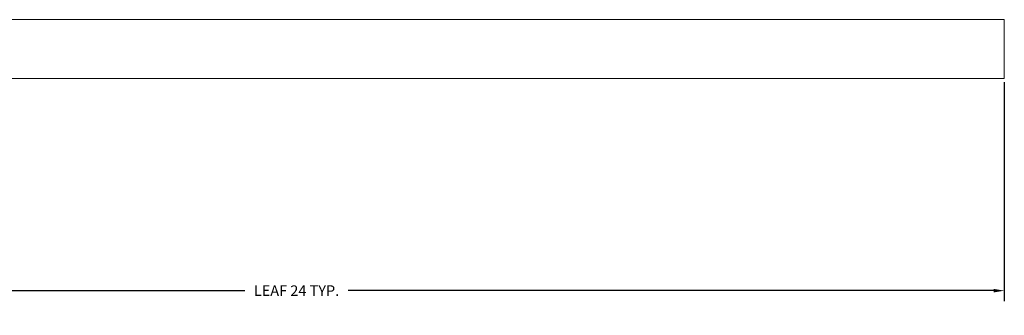
# Model space of a CAD drawing. Units: inches. Extents: x -86 to 2463, y -1058 to 68.
# Tile 7 of 17: x 32.07 to 48.76, y -277.59 to -272.57. Entities that reach past the tile are written whole.
import ezdxf

# ---------------------------------------------------------------- set-up
doc = ezdxf.new("R2010")
doc.units = ezdxf.units.IN
doc.header["$MEASUREMENT"] = 0
doc.layers.add('A-ANNO-DIMS', color=2, linetype='Continuous', lineweight=18)
doc.layers.add('A-DOOR', color=3, linetype='Continuous', lineweight=18)
doc.styles.get("Standard").update_dxf_attribs({"font": 'arial.ttf'})
doc.dimstyles.get("Standard").update_dxf_attribs({"dimtxt": 0.18, "dimasz": 0.18, "dimexe": 0.18, "dimexo": 0.0625, "dimgap": 0.09, "dimtad": 0, "dimtih": 1, "dimtoh": 1, "dimdec": 4, "dimzin": 0, "dimdsep": 46, "dimtxsty": 'Standard', "dimcen": 0.09, "dimadec": 0, "dimazin": 0, "dimtfac": 1, "dimtdec": 4, "dimtofl": 0, "dimtmove": 0, "dimatfit": 3, "dimfxl": 1, "dimtolj": 1, "dimtzin": 0, "dimarcsym": 0})

# ---------------------------------------------------------------- blocks, each defined once
blk = doc.blocks.new('DOOR-LEAF-24IN')
for p, q in [((0, 0), (0, 24)), ((0, 24), (1, 24)), ((1, 24), (1, 0)), ((1, 0), (0, 0))]:
    blk.add_line(p, q)
blk = doc.blocks.new('*D10')
at = {"layer": 'A-ANNO-DIMS', "color": 0, "lineweight": -2, "transparency": 16777216}
for p, q in [((24.761, -273.637), (24.761, -277.354)), ((48.761, -273.637), (48.761, -277.354)), ((24.941, -277.174), (35.887, -277.174)), ((48.581, -277.174), (37.634, -277.174))]:
    blk.add_line(p, q, dxfattribs=at)
at = {"layer": 'A-ANNO-DIMS', "color": 0, "transparency": 16777216}
for points in [[(24.941, -277.144), (24.941, -277.204), (24.761, -277.174)], [(48.581, -277.144), (48.581, -277.204), (48.761, -277.174)]]:
    blk.add_solid(points, dxfattribs=at)
at = {"layer": 'Defpoints', "color": 0, "transparency": 16777216}
for p in [(24.761, -273.574), (48.761, -273.574), (48.761, -277.174)]:
    blk.add_point(p, dxfattribs=at)
at = {"layer": 'A-ANNO-DIMS', "color": 0, "transparency": 16777216, "insert": (36.761, -277.174), "char_height": 0.18, "attachment_point": 5}
blk.add_mtext('\\A1;LEAF 24 TYP.', dxfattribs=at)

msp = doc.modelspace()

# ---------------------------------------------------------------- block references
at = {"layer": 'A-DOOR', "rotation": 270.0000000000001}
msp.add_blockref('DOOR-LEAF-24IN', (24.761, -272.574), dxfattribs=at)

# ---------------------------------------------------------------- dimensions: what is measured, and where the dimension line sits
at = {"layer": 'A-ANNO-DIMS'}
dim = msp.add_linear_dim(base=(48.761, -277.174), p1=(24.761, -273.574), p2=(48.761, -273.574), text='LEAF <> TYP.', dimstyle='Standard', override={"dimdec": 0, "dimlfac": 1, "dimrnd": 0, "dimzin": 0, "dimdsep": 46, "dimlunit": 2}, dxfattribs=at)
dim.commit()
dim.dimension.update_dxf_attribs({"geometry": '*D10', "text_midpoint": (36.761, -277.174)})

doc.saveas('drawing.dxf')
